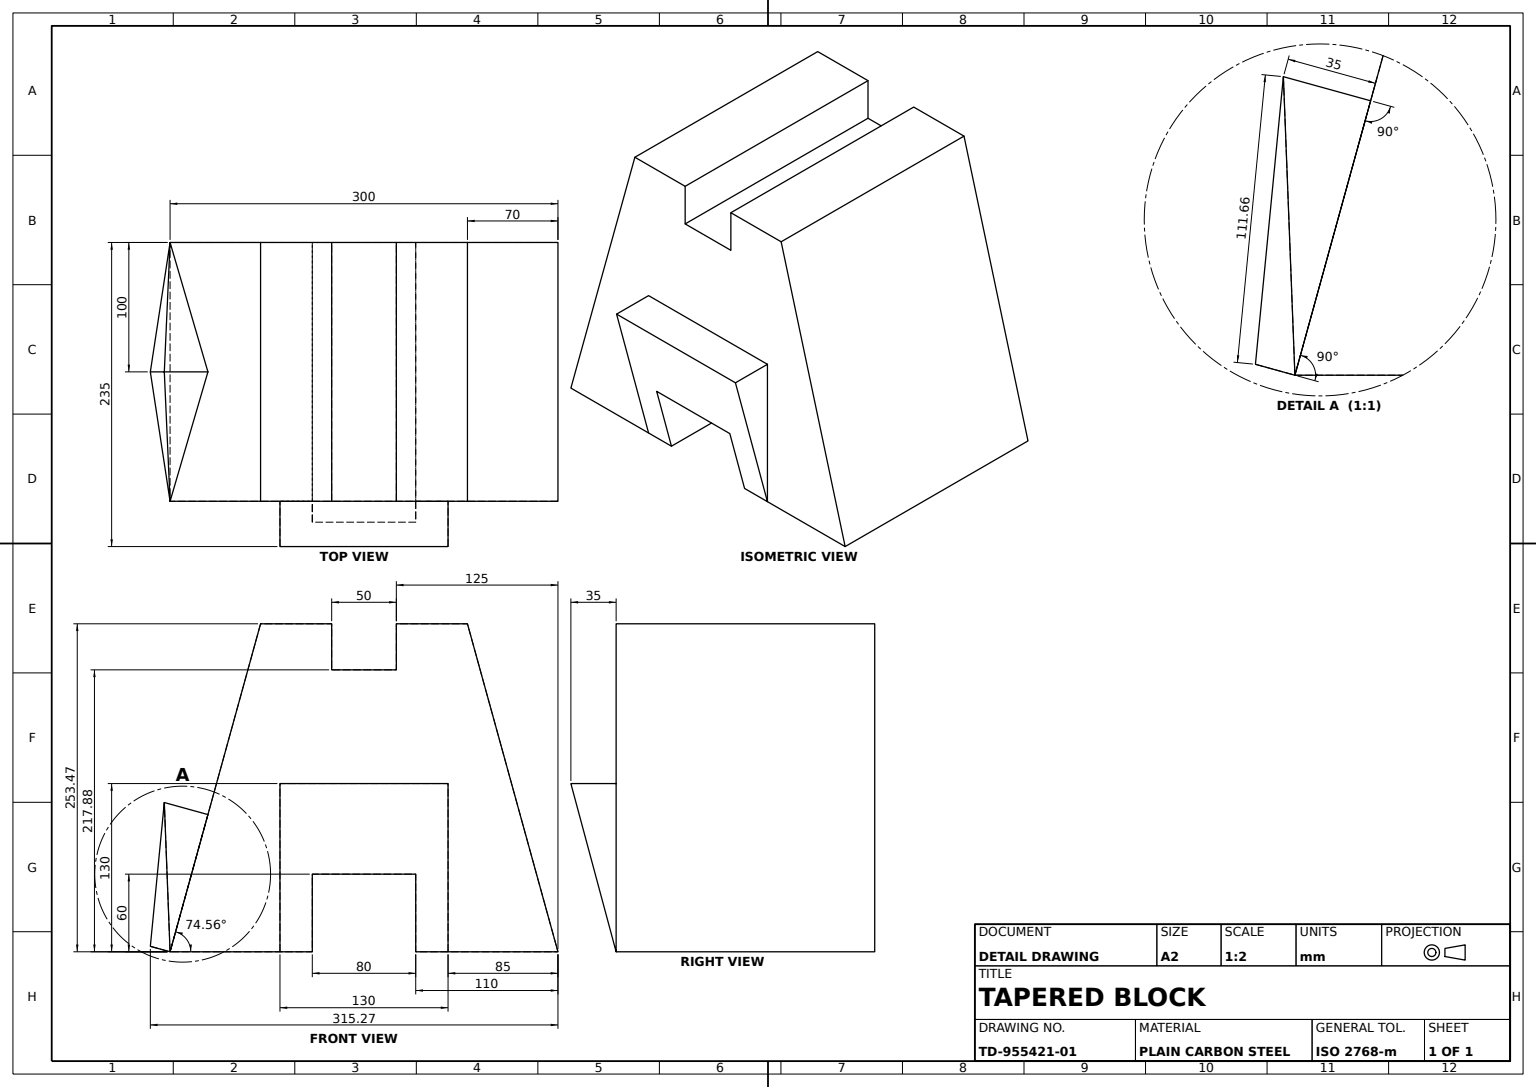
from build123d import *

# Parameters (mm, degrees)
PEDESTAL_BODY_DEPTH  = 100
FRONT_BOSS_DEPTH     = 35
FRONT_BOSS_CUT_DEPTH = 359.742254771
TOP_BOSS_DEPTH       = 35
TOP_BOSS_CUT_A_DEPTH = 324.745166661
TOP_BOSS_CUT_B_DEPTH = 339.016839686


with BuildPart() as part:
    # Pedestal Profile Sketch → Pedestal Body (new, symmetric)
    with BuildSketch(Plane.XY):
        Polygon((40, 0), (40, 60), (-40, 60), (-40, 0), (-150, 0), (-80, 253.467957262), (-25, 253.467957262), (-25, 217.876631195), (25, 217.876631195), (25, 253.467957262), (80, 253.467957262), (150, 0), align=None)
    extrude(amount=PEDESTAL_BODY_DEPTH, both=True)

    # Front Boss Sketch → Front Boss (add)
    with BuildSketch(Plane.XY.offset(100)):
        Polygon((40, 0), (65, 0), (65, 130), (-65, 130), (-65, 0), (-40, 0), (-40, 60), (40, 60), align=None)
    extrude(amount=FRONT_BOSS_DEPTH)

    # Front Boss Cut Sketch → Front Boss Cut (cut, through all)
    with BuildSketch(Plane.ZY.offset(65)):
        Polygon((100, 0), (135, 130), (135, 0), align=None)
    extrude(amount=-FRONT_BOSS_CUT_DEPTH, mode=Mode.SUBTRACT)

    # Top Boss Sketch → Top Boss (add)
    with BuildSketch(Plane(origin=(-139.370318702, 38.489765785, 0), x_dir=(0, 0, 1), z_dir=(-0.9639167277376053, 0.26620394810676146, 0))):
        Polygon((-100, -39.930592216), (0, 70.069407784), (100, -39.930592216), align=None)
    extrude(amount=TOP_BOSS_DEPTH)

    # Top Boss Cut A Sketch → Top Boss Cut A (cut, through all)
    with BuildSketch(Plane(origin=(8.440159726, 30.561572066, 34.87617582), x_dir=(0.9838366716003674, -0.11801541262610508, -0.13467652355552237), z_dir=(0.1790681535458246, 0.6484005584270376, 0.7399400733959439))):
        Polygon((-161.043153096, -65.90530493), (-165.570989176, 86.752805567), (-195.334500882, -58.897918327), align=None)
    extrude(amount=-TOP_BOSS_CUT_A_DEPTH, mode=Mode.SUBTRACT)

    # Top Boss Cut B Sketch → Top Boss Cut B (cut, through all)
    with BuildSketch(Plane(origin=(8.440159726, 30.561572066, -34.87617582), x_dir=(-0.9838366716003674, 0.11801541262610508, -0.13467652355552237), z_dir=(0.1790681535458246, 0.6484005584270376, -0.7399400733959439))):
        Polygon((161.043153096, -65.90530493), (165.570989176, 86.752805567), (192.07604702, -59.563778593), align=None)
    extrude(amount=-TOP_BOSS_CUT_B_DEPTH, mode=Mode.SUBTRACT)


solid = part.part
